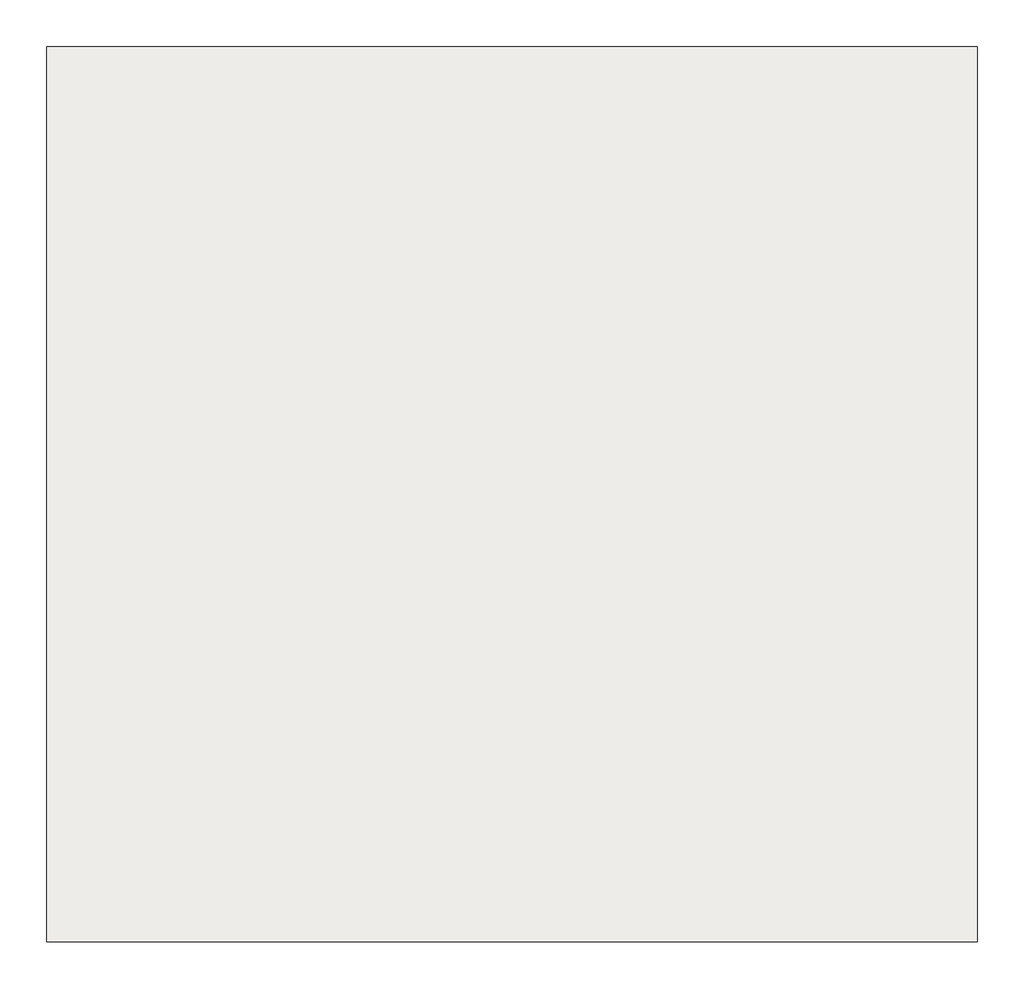
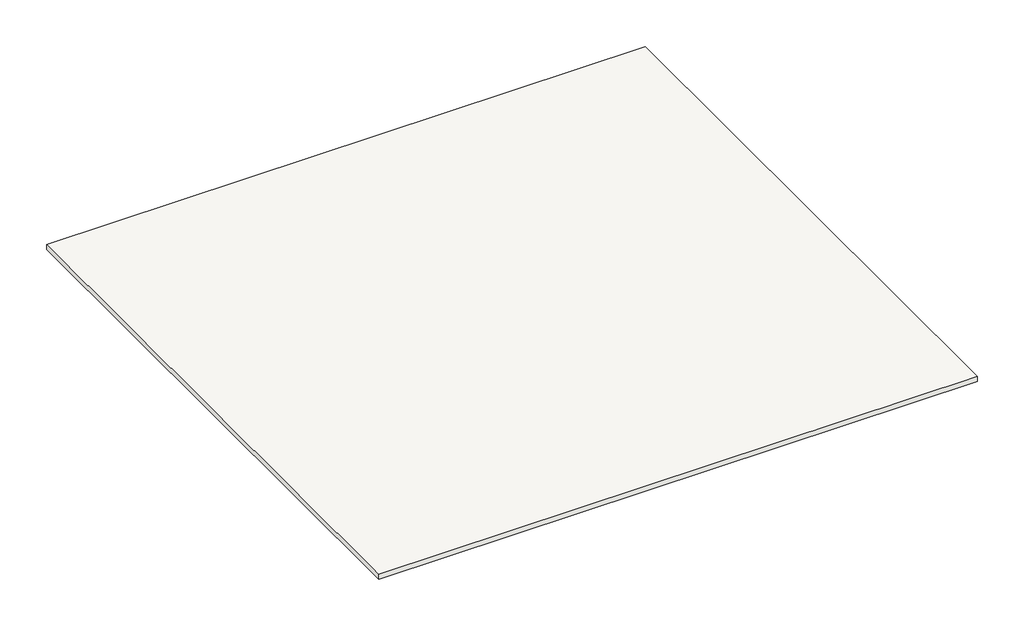
# One storey: 1 slab.
"""IFC4 building model written with IfcOpenShell, lengths in millimetres."""

from ifc_helpers import new_model, si_unit, frame, origin, place, context, project, spatial, polyline, outline, extrude, element, save

model = new_model("IFC4")

# Units and contexts
model_context = context("Model", 3, world=origin())
ifc_project = project(units=[si_unit("LENGTHUNIT", "METRE", prefix="MILLI")], contexts=[model_context])

# Site, building, storey
site = spatial("IfcSite", under=ifc_project)
building = spatial("IfcBuilding", under=site)
storey = spatial("IfcBuildingStorey", under=building, Elevation=15468.6)

# Slab
placement = place(None, origin())
element("IfcSlab", 1, ObjectType="2\"", at=placement, inside=storey, context=model_context, shape_type="SweptSolid", body=[
    extrude(outline(polyline([(3856.5941077, -5525.7354899), (907.1132171, -5525.7354899), (907.1132171, -2688.7252054), (3856.5941077, -2688.7252054), (3856.5941077, -5525.7354899)])), frame((0.0, 0.0, 15443.2), z_axis=(0.0, 0.0, 1.0), x_axis=(1.0, 0.0, 0.0)), (0.0, 0.0, 1.0), 25.4),
])

save(model, "model.ifc")

# Revit data of these elements
# Type "2\""
#   Keynote = "E60/130"
#   Function = 0
#   Layers, outside or top first: 0' - 1" "Concrete, Precast" (function 1)
# Element 1 (IfcSlab, "2\"")
#   Height Offset From Level = 0' - 0"
#   Phase Created = New Construction
#   Materials on its faces: "Concrete, Precast"
# Materials
#   "Concrete, Precast": class "Concrete", colour RGB 192 192 192, transparency 0, Description = "Precast concrete", Cost = 0
